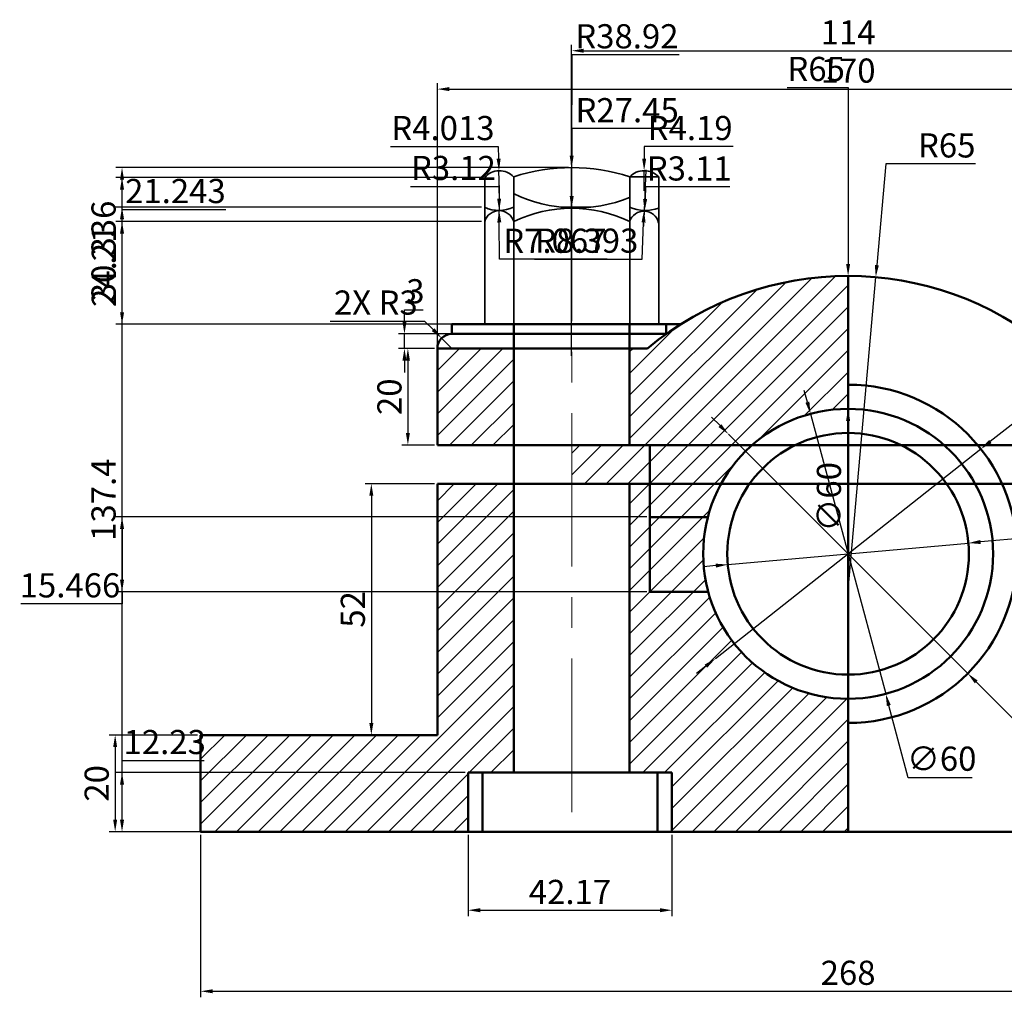
# Model space of a CAD drawing. Units: millimetres. Extents: x 2310 to 2633, y 1180 to 1382.
# Tile 1 of 2: x 2310 to 2514, y 1180 to 1382. Entities that reach past the tile are written whole.
import ezdxf

# ---------------------------------------------------------------- set-up
doc = ezdxf.new("R2010")
doc.units = ezdxf.units.MM
doc.linetypes.add('CENTER', pattern=[50.8, 31.75, -6.35, 6.35, -6.35])
for name, color, linetype, lineweight in [('M-CNTR', 1, 'CENTER', 18), ('M-DIMS', 2, 'Continuous', 25), ('M-FAST', 4, 'Continuous', 35), ('M-HATC', 8, 'Continuous', 18), ('M-OUTL', 7, 'Continuous', 50)]:
    doc.layers.add(name, color=color, linetype=linetype, lineweight=lineweight)
doc.styles.get("Standard").update_dxf_attribs({"font": 'arial.ttf'})
doc.dimstyles.new('ISO-25', dxfattribs={"dimtxt": 5, "dimasz": 2.5, "dimexe": 1.25, "dimexo": 0.625, "dimtad": 1, "dimtoh": 1, "dimdec": 0, "dimtxsty": 'Standard', "dimcen": 2.5, "dimadec": 0, "dimazin": 0, "dimtfac": 1, "dimtdec": 0, "dimtmove": 0, "dimatfit": 3, "dimfxl": 1, "dimarcsym": 0})

# ---------------------------------------------------------------- blocks, each defined once
blk = doc.blocks.new('*D1')
at = {"layer": 'Defpoints', "color": 0, "transparency": 16777216}
for p in [(2538.53, 1375.88), (2424.11, 1351.69), (2538.53, 1351.69)]:
    blk.add_point(p, dxfattribs=at)
at = {"layer": 'M-DIMS', "color": 0, "lineweight": -2, "transparency": 16777216}
for p, q in [((2424.11, 1352.31), (2424.11, 1377.13)), ((2426.61, 1375.88), (2536.03, 1375.88)), ((2538.53, 1352.31), (2538.53, 1377.13))]:
    blk.add_line(p, q, dxfattribs=at)
at = {"layer": 'M-DIMS', "color": 0, "transparency": 16777216}
for points in [[(2426.61, 1376.3), (2426.61, 1375.47), (2424.11, 1375.88)], [(2536.03, 1376.3), (2536.03, 1375.47), (2538.53, 1375.88)]]:
    blk.add_solid(points, dxfattribs=at)
at = {"layer": 'M-DIMS', "color": 0, "transparency": 16777216, "insert": (2481.32, 1379.02), "char_height": 5, "attachment_point": 5}
blk.add_mtext('114', dxfattribs=at)
blk = doc.blocks.new('*D2')
at = {"layer": 'Defpoints', "color": 0, "transparency": 16777216}
for p in [(2347.32, 1214.28), (2615.32, 1214.28), (2615.32, 1181.26)]:
    blk.add_point(p, dxfattribs=at)
at = {"layer": 'M-DIMS', "color": 0, "lineweight": -2, "transparency": 16777216}
for p, q in [((2347.32, 1213.66), (2347.32, 1180.01)), ((2615.32, 1213.66), (2615.32, 1180.01)), ((2349.82, 1181.26), (2612.82, 1181.26))]:
    blk.add_line(p, q, dxfattribs=at)
at = {"layer": 'M-DIMS', "color": 0, "transparency": 16777216}
for points in [[(2349.82, 1181.68), (2349.82, 1180.85), (2347.32, 1181.26)], [(2612.82, 1181.68), (2612.82, 1180.85), (2615.32, 1181.26)]]:
    blk.add_solid(points, dxfattribs=at)
at = {"layer": 'M-DIMS', "color": 0, "transparency": 16777216, "insert": (2481.32, 1184.44), "char_height": 5, "attachment_point": 5}
blk.add_mtext('268', dxfattribs=at)
blk = doc.blocks.new('*D3')
at = {"layer": 'Defpoints', "color": 0, "transparency": 16777216}
for p in [(2396.32, 1314.28), (2390.22, 1294.28), (2396.32, 1294.28)]:
    blk.add_point(p, dxfattribs=at)
at = {"layer": 'M-DIMS', "color": 0, "lineweight": -2, "transparency": 16777216}
for p, q in [((2395.7, 1314.28), (2388.97, 1314.28)), ((2390.22, 1311.78), (2390.22, 1296.78)), ((2395.7, 1294.28), (2388.97, 1294.28))]:
    blk.add_line(p, q, dxfattribs=at)
at = {"layer": 'M-DIMS', "color": 0, "transparency": 16777216}
for points in [[(2389.81, 1311.78), (2390.64, 1311.78), (2390.22, 1314.28)], [(2389.81, 1296.78), (2390.64, 1296.78), (2390.22, 1294.28)]]:
    blk.add_solid(points, dxfattribs=at)
at = {"layer": 'M-DIMS', "color": 0, "transparency": 16777216, "insert": (2387.05, 1304.28), "char_height": 5, "attachment_point": 5, "rotation": 90}
blk.add_mtext('20', dxfattribs=at)
blk = doc.blocks.new('*D4')
at = {"layer": 'Defpoints', "color": 0, "transparency": 16777216}
for p in [(2396.32, 1286.28), (2382.66, 1234.28), (2396.32, 1234.28)]:
    blk.add_point(p, dxfattribs=at)
at = {"layer": 'M-DIMS', "color": 0, "lineweight": -2, "transparency": 16777216}
for p, q in [((2395.7, 1286.28), (2381.41, 1286.28)), ((2382.66, 1283.78), (2382.66, 1236.78)), ((2395.7, 1234.28), (2381.41, 1234.28))]:
    blk.add_line(p, q, dxfattribs=at)
at = {"layer": 'M-DIMS', "color": 0, "transparency": 16777216}
for points in [[(2382.24, 1283.78), (2383.08, 1283.78), (2382.66, 1286.28)], [(2382.24, 1236.78), (2383.08, 1236.78), (2382.66, 1234.28)]]:
    blk.add_solid(points, dxfattribs=at)
at = {"layer": 'M-DIMS', "color": 0, "transparency": 16777216, "insert": (2379.48, 1260.28), "char_height": 5, "attachment_point": 5, "rotation": 90}
blk.add_mtext('52', dxfattribs=at)
blk = doc.blocks.new('*D5')
at = {"layer": 'Defpoints', "color": 0, "transparency": 16777216}
for p in [(2347.32, 1234.28), (2329.65, 1214.28), (2347.32, 1214.28)]:
    blk.add_point(p, dxfattribs=at)
at = {"layer": 'M-DIMS', "color": 0, "lineweight": -2, "transparency": 16777216}
for p, q in [((2346.7, 1234.28), (2328.4, 1234.28)), ((2329.65, 1231.78), (2329.65, 1216.78)), ((2346.7, 1214.28), (2328.4, 1214.28))]:
    blk.add_line(p, q, dxfattribs=at)
at = {"layer": 'M-DIMS', "color": 0, "transparency": 16777216}
for points in [[(2329.23, 1231.78), (2330.06, 1231.78), (2329.65, 1234.28)], [(2329.23, 1216.78), (2330.06, 1216.78), (2329.65, 1214.28)]]:
    blk.add_solid(points, dxfattribs=at)
at = {"layer": 'M-DIMS', "color": 0, "transparency": 16777216, "insert": (2326.47, 1224.28), "char_height": 5, "attachment_point": 5, "rotation": 90}
blk.add_mtext('20', dxfattribs=at)
blk = doc.blocks.new('*D6')
at = {"layer": 'Defpoints', "color": 0, "transparency": 16777216}
for p in [(2389.51, 1317.28), (2399.32, 1317.28), (2396.32, 1314.28)]:
    blk.add_point(p, dxfattribs=at)
at = {"layer": 'M-DIMS', "color": 0, "lineweight": -2, "transparency": 16777216}
for p, q in [((2389.51, 1319.78), (2389.51, 1322.28)), ((2389.51, 1322.28), (2393.41, 1322.28)), ((2398.7, 1317.28), (2388.26, 1317.28)), ((2389.51, 1314.28), (2389.51, 1317.28)), ((2395.7, 1314.28), (2388.26, 1314.28)), ((2389.51, 1311.78), (2389.51, 1309.28))]:
    blk.add_line(p, q, dxfattribs=at)
at = {"layer": 'M-DIMS', "color": 0, "transparency": 16777216}
for points in [[(2389.1, 1319.78), (2389.93, 1319.78), (2389.51, 1317.28)], [(2389.1, 1311.78), (2389.93, 1311.78), (2389.51, 1314.28)]]:
    blk.add_solid(points, dxfattribs=at)
at = {"layer": 'M-DIMS', "color": 0, "transparency": 16777216, "insert": (2391.78, 1325.46), "char_height": 5, "attachment_point": 5}
blk.add_mtext('3', dxfattribs=at)
blk = doc.blocks.new('*D8')
at = {"layer": 'Defpoints', "color": 0, "transparency": 16777216}
for p in [(2487.04, 1329.03), (2481.32, 1264.28)]:
    blk.add_point(p, dxfattribs=at)
at = {"layer": 'M-DIMS', "color": 0, "lineweight": -2, "transparency": 16777216}
for p, q in [((2489.11, 1352.46), (2487.26, 1331.52)), ((2507.71, 1352.46), (2489.11, 1352.46)), ((2481.32, 1264.28), (2487.04, 1329.03))]:
    blk.add_line(p, q, dxfattribs=at)
at = {"layer": 'M-DIMS', "color": 0, "transparency": 16777216}
blk.add_solid([(2486.85, 1331.56), (2487.68, 1331.48), (2487.04, 1329.03)], dxfattribs=at)
at = {"layer": 'M-DIMS', "color": 0, "transparency": 16777216, "insert": (2501.72, 1355.64), "char_height": 5, "attachment_point": 5}
blk.add_mtext('R65', dxfattribs=at)
blk = doc.blocks.new('*D9')
at = {"layer": 'Defpoints', "color": 0, "transparency": 16777216}
for p in [(2508.79, 1293.47), (2453.85, 1250.09)]:
    blk.add_point(p, dxfattribs=at)
at = {"layer": 'M-DIMS', "color": 0, "lineweight": -2, "transparency": 16777216}
for p, q in [((2516.9, 1299.87), (2510.75, 1295.02)), ((2536.4, 1299.87), (2516.9, 1299.87)), ((2453.85, 1250.09), (2508.79, 1293.47)), ((2451.89, 1248.54), (2449.93, 1246.99))]:
    blk.add_line(p, q, dxfattribs=at)
at = {"layer": 'M-DIMS', "color": 0, "transparency": 16777216}
for points in [[(2510.49, 1295.35), (2511.01, 1294.69), (2508.79, 1293.47)], [(2451.63, 1248.87), (2452.15, 1248.21), (2453.85, 1250.09)]]:
    blk.add_solid(points, dxfattribs=at)
at = {"layer": 'M-DIMS', "color": 0, "transparency": 16777216, "insert": (2530.11, 1303.19), "char_height": 5, "attachment_point": 5}
blk.add_mtext('∅70', dxfattribs=at)
blk = doc.blocks.new('*D10')
at = {"layer": 'Defpoints', "color": 0, "transparency": 16777216}
for p in [(2481.32, 1301.78), (2481.32, 1241.78)]:
    blk.add_point(p, dxfattribs=at)
at = {"layer": 'M-DIMS', "color": 0, "lineweight": -2, "transparency": 16777216}
blk.add_line((2481.32, 1276.65), (2481.32, 1299.28), dxfattribs=at)
at = {"layer": 'M-DIMS', "color": 0, "transparency": 16777216}
blk.add_solid([(2480.9, 1299.28), (2481.74, 1299.28), (2481.32, 1301.78)], dxfattribs=at)
at = {"layer": 'M-DIMS', "color": 0, "transparency": 16777216, "insert": (2478, 1283.57), "char_height": 5, "attachment_point": 5, "rotation": 90}
blk.add_mtext('∅60', dxfattribs=at)
blk = doc.blocks.new('*D11')
at = {"layer": 'Defpoints', "color": 0, "transparency": 16777216}
for p in [(2506.22, 1274.01), (2456.42, 1269.55)]:
    blk.add_point(p, dxfattribs=at)
at = {"layer": 'M-DIMS', "color": 0, "lineweight": -2, "transparency": 16777216}
for p, q in [((2456.42, 1269.55), (2506.22, 1274.01)), ((2520.89, 1275.32), (2508.71, 1274.23)), ((2534.1, 1275.32), (2520.89, 1275.32)), ((2453.93, 1269.33), (2451.44, 1269.11))]:
    blk.add_line(p, q, dxfattribs=at)
at = {"layer": 'M-DIMS', "color": 0, "transparency": 16777216}
for points in [[(2508.68, 1274.64), (2508.75, 1273.81), (2506.22, 1274.01)], [(2453.89, 1269.75), (2453.97, 1268.92), (2456.42, 1269.55)]]:
    blk.add_solid(points, dxfattribs=at)
at = {"layer": 'M-DIMS', "color": 0, "transparency": 16777216, "insert": (2527.81, 1278.64), "char_height": 5, "attachment_point": 5}
blk.add_mtext('∅50', dxfattribs=at)
blk = doc.blocks.new('HEX-NUT-M16')
for p, q in [((0.01, 21.24), (0.01, 30.34)), ((6.01, 27.03), (6.01, 30.51)), ((30.01, 30.51), (36.01, 30.51)), ((30.01, 28.24), (30.01, 30.51)), ((36.01, 28), (36.01, 30.51)), ((6.01, 24.24), (6.01, 27.03)), ((30.01, 24.24), (30.01, 28.24)), ((36.01, 24), (36.01, 28)), ((6.01, 21.24), (6.01, 24.24)), ((22, 24.24), (15.78, 24.24)), ((30.01, 21.24), (30.01, 24.24)), ((36.01, 21), (36.01, 24)), ((0.01, 0), (0.01, 21.24)), ((6.01, 21.24), (6.01, 0)), ((30.01, 21.24), (30.01, 0)), ((36.01, 0), (36.01, 21)), ((6.01, 0), (0.01, 0)), ((30.01, 0), (36.01, 0))]:
    blk.add_line(p, q)
for centre, radius, start, end in [((3.08, 27.76), 4.01, 43.2858, 140.0947), ((18.01, -6.51), 38.92, 72.0429, 107.9571), ((33.01, 27.59), 4.19, 44.2799, 135.7201), ((18.89, 53.7), 29.62, 244.2052, 292.0376), ((2.96, 30.62), 7.07, 245.1977, 295.4854), ((3.01, 20.39), 3.12, 15.8422, 164.1674), ((18.01, -3.45), 27.45, 64.08, 115.92), ((33.32, 31.95), 8.39, 246.714, 288.6385), ((32.97, 20.31), 3.11, 12.8097, 162.5427)]:
    blk.add_arc(centre, radius, start, end)
blk = doc.blocks.new('*D13')
at = {"layer": 'Defpoints', "color": 0, "transparency": 16777216}
for p in [(2566.32, 1367.94), (2396.32, 1314.28), (2566.32, 1314.28)]:
    blk.add_point(p, dxfattribs=at)
at = {"layer": 'M-DIMS', "color": 0, "lineweight": -2, "transparency": 16777216}
for p, q in [((2396.32, 1314.91), (2396.32, 1369.19)), ((2398.82, 1367.94), (2563.82, 1367.94)), ((2566.32, 1314.91), (2566.32, 1369.19))]:
    blk.add_line(p, q, dxfattribs=at)
at = {"layer": 'M-DIMS', "color": 0, "transparency": 16777216}
for points in [[(2398.82, 1368.36), (2398.82, 1367.52), (2396.32, 1367.94)], [(2563.82, 1368.36), (2563.82, 1367.52), (2566.32, 1367.94)]]:
    blk.add_solid(points, dxfattribs=at)
at = {"layer": 'M-DIMS', "color": 0, "transparency": 16777216, "insert": (2481.32, 1371.12), "char_height": 5, "attachment_point": 5}
blk.add_mtext('170', dxfattribs=at)
blk = doc.blocks.new('*D16')
at = {"layer": 'Defpoints', "color": 0, "transparency": 16777216}
for p in [(2331.07, 1351.69), (2424.11, 1351.69), (2347.32, 1214.28)]:
    blk.add_point(p, dxfattribs=at)
at = {"layer": 'M-DIMS', "color": 0, "lineweight": -2, "transparency": 16777216}
for p, q in [((2423.49, 1351.69), (2329.82, 1351.69)), ((2331.07, 1216.78), (2331.07, 1349.19)), ((2346.7, 1214.28), (2329.82, 1214.28))]:
    blk.add_line(p, q, dxfattribs=at)
at = {"layer": 'M-DIMS', "color": 0, "transparency": 16777216}
for points in [[(2330.65, 1349.19), (2331.49, 1349.19), (2331.07, 1351.69)], [(2330.65, 1216.78), (2331.49, 1216.78), (2331.07, 1214.28)]]:
    blk.add_solid(points, dxfattribs=at)
at = {"layer": 'M-DIMS', "color": 0, "transparency": 16777216, "insert": (2327.89, 1282.98), "char_height": 5, "attachment_point": 5, "rotation": 90}
blk.add_mtext('137.4', dxfattribs=at)
blk = doc.blocks.new('*D17')
at = {"layer": 'Defpoints', "color": 0, "transparency": 16777216}
for p in [(2402.68, 1214.28), (2444.86, 1214.28), (2444.86, 1198.03)]:
    blk.add_point(p, dxfattribs=at)
at = {"layer": 'M-DIMS', "color": 0, "lineweight": -2, "transparency": 16777216}
for p, q in [((2402.68, 1213.66), (2402.68, 1196.78)), ((2444.86, 1213.66), (2444.86, 1196.78)), ((2405.18, 1198.03), (2442.36, 1198.03))]:
    blk.add_line(p, q, dxfattribs=at)
at = {"layer": 'M-DIMS', "color": 0, "transparency": 16777216}
for points in [[(2405.18, 1198.45), (2405.18, 1197.61), (2402.68, 1198.03)], [(2442.36, 1198.45), (2442.36, 1197.61), (2444.86, 1198.03)]]:
    blk.add_solid(points, dxfattribs=at)
at = {"layer": 'M-DIMS', "color": 0, "transparency": 16777216, "insert": (2423.77, 1201.17), "char_height": 5, "attachment_point": 5}
blk.add_mtext('42.17', dxfattribs=at)
blk = doc.blocks.new('*D18')
at = {"layer": 'Defpoints', "color": 0, "transparency": 16777216}
for p in [(2331.07, 1226.51), (2402.68, 1226.51), (2402.68, 1214.28)]:
    blk.add_point(p, dxfattribs=at)
at = {"layer": 'M-DIMS', "color": 0, "lineweight": -2, "transparency": 16777216}
for p, q in [((2331.07, 1226.51), (2331.07, 1229.01)), ((2331.07, 1229.01), (2348.1, 1229.01)), ((2402.06, 1226.51), (2329.82, 1226.51)), ((2331.07, 1216.78), (2331.07, 1224.01)), ((2402.06, 1214.28), (2329.82, 1214.28))]:
    blk.add_line(p, q, dxfattribs=at)
at = {"layer": 'M-DIMS', "color": 0, "transparency": 16777216}
for points in [[(2330.65, 1224.01), (2331.49, 1224.01), (2331.07, 1226.51)], [(2330.65, 1216.78), (2331.49, 1216.78), (2331.07, 1214.28)]]:
    blk.add_solid(points, dxfattribs=at)
at = {"layer": 'M-DIMS', "color": 0, "transparency": 16777216, "insert": (2339.9, 1232.19), "char_height": 5, "attachment_point": 5}
blk.add_mtext('12.23', dxfattribs=at)
blk = doc.blocks.new('*D19')
at = {"layer": 'Defpoints', "color": 0, "transparency": 16777216}
for p in [(2473.54, 1300.75), (2489.1, 1242.81)]:
    blk.add_point(p, dxfattribs=at)
at = {"layer": 'M-DIMS', "color": 0, "lineweight": -2, "transparency": 16777216}
for p, q in [((2472.9, 1303.17), (2472.25, 1305.58)), ((2473.54, 1300.75), (2489.1, 1242.81)), ((2493.76, 1225.42), (2489.75, 1240.39)), ((2506.97, 1225.42), (2493.76, 1225.42))]:
    blk.add_line(p, q, dxfattribs=at)
at = {"layer": 'M-DIMS', "color": 0, "transparency": 16777216}
for points in [[(2473.3, 1303.28), (2472.49, 1303.06), (2473.54, 1300.75)], [(2490.15, 1240.5), (2489.34, 1240.28), (2489.1, 1242.81)]]:
    blk.add_solid(points, dxfattribs=at)
at = {"layer": 'M-DIMS', "color": 0, "transparency": 16777216, "insert": (2500.68, 1228.74), "char_height": 5, "attachment_point": 5}
blk.add_mtext('∅60', dxfattribs=at)
blk = doc.blocks.new('*D20')
at = {"layer": 'Defpoints', "color": 0, "transparency": 16777216}
for p in [(2456.57, 1296.53), (2506.07, 1247.03)]:
    blk.add_point(p, dxfattribs=at)
at = {"layer": 'M-DIMS', "color": 0, "lineweight": -2, "transparency": 16777216}
for p, q in [((2454.81, 1298.3), (2453.04, 1300.07)), ((2456.57, 1296.53), (2506.07, 1247.03)), ((2520.92, 1232.18), (2507.84, 1245.26)), ((2534.13, 1232.18), (2520.92, 1232.18))]:
    blk.add_line(p, q, dxfattribs=at)
at = {"layer": 'M-DIMS', "color": 0, "transparency": 16777216}
for points in [[(2455.1, 1298.59), (2454.51, 1298), (2456.57, 1296.53)], [(2508.13, 1245.56), (2507.54, 1244.97), (2506.07, 1247.03)]]:
    blk.add_solid(points, dxfattribs=at)
at = {"layer": 'M-DIMS', "color": 0, "transparency": 16777216, "insert": (2527.84, 1235.5), "char_height": 5, "attachment_point": 5}
blk.add_mtext('∅70', dxfattribs=at)
blk = doc.blocks.new('*D21')
at = {"layer": 'Defpoints', "color": 0, "transparency": 16777216}
for p in [(2481.32, 1329.28), (2481.32, 1264.28)]:
    blk.add_point(p, dxfattribs=at)
at = {"layer": 'M-DIMS', "color": 0, "lineweight": -2, "transparency": 16777216}
for p, q in [((2468.71, 1368.28), (2481.32, 1368.28)), ((2481.32, 1368.28), (2481.32, 1331.78)), ((2481.32, 1264.28), (2481.32, 1329.28))]:
    blk.add_line(p, q, dxfattribs=at)
at = {"layer": 'M-DIMS', "color": 0, "transparency": 16777216}
blk.add_solid([(2481.74, 1331.78), (2480.9, 1331.78), (2481.32, 1329.28)], dxfattribs=at)
at = {"layer": 'M-DIMS', "color": 0, "transparency": 16777216, "insert": (2474.7, 1371.46), "char_height": 5, "attachment_point": 5}
blk.add_mtext('R65', dxfattribs=at)
blk = doc.blocks.new('*D23')
at = {"layer": 'Defpoints', "color": 0, "transparency": 16777216}
for p in [(2397.2, 1316.4), (2399.32, 1314.28)]:
    blk.add_point(p, dxfattribs=at)
at = {"layer": 'M-DIMS', "color": 0, "lineweight": -2, "transparency": 16777216}
for p, q in [((2374.15, 1319.94), (2393.66, 1319.94)), ((2393.66, 1319.94), (2395.43, 1318.17)), ((2399.32, 1314.28), (2397.2, 1316.4))]:
    blk.add_line(p, q, dxfattribs=at)
at = {"layer": 'M-DIMS', "color": 0, "transparency": 16777216}
blk.add_solid([(2395.73, 1318.46), (2395.14, 1317.88), (2397.2, 1316.4)], dxfattribs=at)
at = {"layer": 'M-DIMS', "color": 0, "transparency": 16777216, "insert": (2383.59, 1323.12), "char_height": 5, "attachment_point": 5}
blk.add_mtext('2X R3', dxfattribs=at)
blk = doc.blocks.new('*D25')
at = {"layer": 'Defpoints', "color": 0, "transparency": 16777216}
for p in [(2331.07, 1340.52), (2406.11, 1340.52), (2406.11, 1319.28)]:
    blk.add_point(p, dxfattribs=at)
at = {"layer": 'M-DIMS', "color": 0, "lineweight": -2, "transparency": 16777216}
for p, q in [((2331.07, 1340.52), (2331.07, 1343.02)), ((2331.07, 1343.02), (2352.54, 1343.02)), ((2405.49, 1340.52), (2329.82, 1340.52)), ((2331.07, 1321.78), (2331.07, 1338.02)), ((2405.49, 1319.28), (2329.82, 1319.28))]:
    blk.add_line(p, q, dxfattribs=at)
at = {"layer": 'M-DIMS', "color": 0, "transparency": 16777216}
for points in [[(2330.65, 1338.02), (2331.49, 1338.02), (2331.07, 1340.52)], [(2330.65, 1321.78), (2331.49, 1321.78), (2331.07, 1319.28)]]:
    blk.add_solid(points, dxfattribs=at)
at = {"layer": 'M-DIMS', "color": 0, "transparency": 16777216, "insert": (2342.12, 1346.2), "char_height": 5, "attachment_point": 5}
blk.add_mtext('21.243', dxfattribs=at)
blk = doc.blocks.new('*D26')
at = {"layer": 'Defpoints', "color": 0, "transparency": 16777216}
for p in [(2331.07, 1343.49), (2406.11, 1343.49), (2406.11, 1319.28)]:
    blk.add_point(p, dxfattribs=at)
at = {"layer": 'M-DIMS', "color": 0, "lineweight": -2, "transparency": 16777216}
for p, q in [((2405.48, 1343.49), (2329.82, 1343.49)), ((2331.07, 1321.78), (2331.07, 1340.99)), ((2405.49, 1319.28), (2329.82, 1319.28))]:
    blk.add_line(p, q, dxfattribs=at)
at = {"layer": 'M-DIMS', "color": 0, "transparency": 16777216}
for points in [[(2330.65, 1340.99), (2331.49, 1340.99), (2331.07, 1343.49)], [(2330.65, 1321.78), (2331.49, 1321.78), (2331.07, 1319.28)]]:
    blk.add_solid(points, dxfattribs=at)
at = {"layer": 'M-DIMS', "color": 0, "transparency": 16777216, "insert": (2327.94, 1331.38), "char_height": 5, "attachment_point": 5, "rotation": 90}
blk.add_mtext('24.21', dxfattribs=at)
blk = doc.blocks.new('*D27')
at = {"layer": 'Defpoints', "color": 0, "transparency": 16777216}
for p in [(2331.07, 1349.62), (2406.11, 1349.62), (2406.11, 1319.28)]:
    blk.add_point(p, dxfattribs=at)
at = {"layer": 'M-DIMS', "color": 0, "lineweight": -2, "transparency": 16777216}
for p, q in [((2405.49, 1349.62), (2329.82, 1349.62)), ((2331.07, 1321.78), (2331.07, 1347.12)), ((2405.49, 1319.28), (2329.82, 1319.28))]:
    blk.add_line(p, q, dxfattribs=at)
at = {"layer": 'M-DIMS', "color": 0, "transparency": 16777216}
for points in [[(2330.65, 1347.12), (2331.49, 1347.12), (2331.07, 1349.62)], [(2330.65, 1321.78), (2331.49, 1321.78), (2331.07, 1319.28)]]:
    blk.add_solid(points, dxfattribs=at)
at = {"layer": 'M-DIMS', "color": 0, "transparency": 16777216, "insert": (2327.89, 1334.45), "char_height": 5, "attachment_point": 5, "rotation": 90}
blk.add_mtext('30.336', dxfattribs=at)
blk = doc.blocks.new('*D28')
at = {"layer": 'Defpoints', "color": 0, "transparency": 16777216}
for p in [(2440.28, 1279.4), (2331.07, 1263.93), (2440.28, 1263.93)]:
    blk.add_point(p, dxfattribs=at)
at = {"layer": 'M-DIMS', "color": 0, "lineweight": -2, "transparency": 16777216}
for p, q in [((2439.65, 1279.4), (2329.82, 1279.4)), ((2331.07, 1276.9), (2331.07, 1266.43)), ((2439.65, 1263.93), (2329.82, 1263.93)), ((2331.07, 1263.93), (2331.07, 1261.43)), ((2331.07, 1261.43), (2310.16, 1261.43))]:
    blk.add_line(p, q, dxfattribs=at)
at = {"layer": 'M-DIMS', "color": 0, "transparency": 16777216}
for points in [[(2330.65, 1276.9), (2331.49, 1276.9), (2331.07, 1279.4)], [(2330.65, 1266.43), (2331.49, 1266.43), (2331.07, 1263.93)]]:
    blk.add_solid(points, dxfattribs=at)
at = {"layer": 'M-DIMS', "color": 0, "transparency": 16777216, "insert": (2320.3, 1264.61), "char_height": 5, "attachment_point": 5}
blk.add_mtext('15.466', dxfattribs=at)
blk = doc.blocks.new('*D29')
at = {"layer": 'Defpoints', "color": 0, "transparency": 16777216}
for p in [(2424.11, 1351.69), (2424.11, 1312.77)]:
    blk.add_point(p, dxfattribs=at)
at = {"layer": 'M-DIMS', "color": 0, "lineweight": -2, "transparency": 16777216}
for p, q in [((2446.35, 1375.04), (2424.12, 1375.04)), ((2424.12, 1375.04), (2424.11, 1354.19)), ((2424.11, 1312.77), (2424.11, 1351.69))]:
    blk.add_line(p, q, dxfattribs=at)
at = {"layer": 'M-DIMS', "color": 0, "transparency": 16777216}
blk.add_solid([(2423.7, 1354.19), (2424.53, 1354.19), (2424.11, 1351.69)], dxfattribs=at)
at = {"layer": 'M-DIMS', "color": 0, "transparency": 16777216, "insert": (2435.54, 1378.22), "char_height": 5, "attachment_point": 5}
blk.add_mtext('R38.92', dxfattribs=at)
blk = doc.blocks.new('*D30')
at = {"layer": 'Defpoints', "color": 0, "transparency": 16777216}
for p in [(2424.11, 1343.29), (2424.11, 1315.83)]:
    blk.add_point(p, dxfattribs=at)
at = {"layer": 'M-DIMS', "color": 0, "lineweight": -2, "transparency": 16777216}
for p, q in [((2446.44, 1359.76), (2424.12, 1359.76)), ((2424.12, 1359.76), (2424.11, 1345.79)), ((2424.11, 1315.83), (2424.11, 1343.29))]:
    blk.add_line(p, q, dxfattribs=at)
at = {"layer": 'M-DIMS', "color": 0, "transparency": 16777216}
blk.add_solid([(2423.7, 1345.79), (2424.53, 1345.79), (2424.11, 1343.29)], dxfattribs=at)
at = {"layer": 'M-DIMS', "color": 0, "transparency": 16777216, "insert": (2435.59, 1362.93), "char_height": 5, "attachment_point": 5}
blk.add_mtext('R27.45', dxfattribs=at)
blk = doc.blocks.new('*D31')
at = {"layer": 'Defpoints', "color": 0, "transparency": 16777216}
for p in [(2439.43, 1351.23), (2439.09, 1342.85)]:
    blk.add_point(p, dxfattribs=at)
at = {"layer": 'M-DIMS', "color": 0, "lineweight": -2, "transparency": 16777216}
for p, q in [((2439.43, 1351.23), (2439.09, 1342.85)), ((2438.68, 1332.75), (2438.99, 1340.35)), ((2416.4, 1332.75), (2438.68, 1332.75))]:
    blk.add_line(p, q, dxfattribs=at)
at = {"layer": 'M-DIMS', "color": 0, "transparency": 16777216}
blk.add_solid([(2438.57, 1340.37), (2439.41, 1340.33), (2439.09, 1342.85)], dxfattribs=at)
at = {"layer": 'M-DIMS', "color": 0, "transparency": 16777216, "insert": (2427.23, 1335.93), "char_height": 5, "attachment_point": 5}
blk.add_mtext('R8.393', dxfattribs=at)
blk = doc.blocks.new('*D32')
at = {"layer": 'Defpoints', "color": 0, "transparency": 16777216}
for p in [(2409.07, 1349.9), (2409.12, 1342.84)]:
    blk.add_point(p, dxfattribs=at)
at = {"layer": 'M-DIMS', "color": 0, "lineweight": -2, "transparency": 16777216}
for p, q in [((2409.07, 1349.9), (2409.12, 1342.84)), ((2409.18, 1332.73), (2409.13, 1340.34)), ((2431.46, 1332.73), (2409.18, 1332.73))]:
    blk.add_line(p, q, dxfattribs=at)
at = {"layer": 'M-DIMS', "color": 0, "transparency": 16777216}
blk.add_solid([(2409.55, 1340.34), (2408.71, 1340.33), (2409.12, 1342.84)], dxfattribs=at)
at = {"layer": 'M-DIMS', "color": 0, "transparency": 16777216, "insert": (2420.63, 1335.91), "char_height": 5, "attachment_point": 5}
blk.add_mtext('R7.067', dxfattribs=at)
blk = doc.blocks.new('*D33')
at = {"layer": 'Defpoints', "color": 0, "transparency": 16777216}
for p in [(2439.11, 1351.06), (2439.11, 1346.87)]:
    blk.add_point(p, dxfattribs=at)
at = {"layer": 'M-DIMS', "color": 0, "lineweight": -2, "transparency": 16777216}
for p, q in [((2457.52, 1356.06), (2439.12, 1356.06)), ((2439.12, 1356.06), (2439.12, 1353.56)), ((2439.11, 1346.87), (2439.11, 1351.06))]:
    blk.add_line(p, q, dxfattribs=at)
at = {"layer": 'M-DIMS', "color": 0, "transparency": 16777216}
blk.add_solid([(2438.7, 1353.56), (2439.53, 1353.56), (2439.11, 1351.06)], dxfattribs=at)
at = {"layer": 'M-DIMS', "color": 0, "transparency": 16777216, "insert": (2448.63, 1359.24), "char_height": 5, "attachment_point": 5}
blk.add_mtext('R4.19', dxfattribs=at)
blk = doc.blocks.new('*D34')
at = {"layer": 'Defpoints', "color": 0, "transparency": 16777216}
for p in [(2409.07, 1351.05), (2409.19, 1347.04)]:
    blk.add_point(p, dxfattribs=at)
at = {"layer": 'M-DIMS', "color": 0, "lineweight": -2, "transparency": 16777216}
for p, q in [((2386.65, 1356.05), (2408.93, 1356.05)), ((2408.93, 1356.05), (2409, 1353.55)), ((2409.19, 1347.04), (2409.07, 1351.05))]:
    blk.add_line(p, q, dxfattribs=at)
at = {"layer": 'M-DIMS', "color": 0, "transparency": 16777216}
blk.add_solid([(2409.42, 1353.56), (2408.58, 1353.54), (2409.07, 1351.05)], dxfattribs=at)
at = {"layer": 'M-DIMS', "color": 0, "transparency": 16777216, "insert": (2397.47, 1359.23), "char_height": 5, "attachment_point": 5}
blk.add_mtext('R4.013', dxfattribs=at)
blk = doc.blocks.new('*D35')
at = {"layer": 'Defpoints', "color": 0, "transparency": 16777216}
for p in [(2409.11, 1342.79), (2409.11, 1339.67)]:
    blk.add_point(p, dxfattribs=at)
at = {"layer": 'M-DIMS', "color": 0, "lineweight": -2, "transparency": 16777216}
for p, q in [((2390.77, 1347.79), (2409.11, 1347.79)), ((2409.11, 1347.79), (2409.11, 1345.29)), ((2409.11, 1339.67), (2409.11, 1342.79))]:
    blk.add_line(p, q, dxfattribs=at)
at = {"layer": 'M-DIMS', "color": 0, "transparency": 16777216}
blk.add_solid([(2409.53, 1345.29), (2408.7, 1345.29), (2409.11, 1342.79)], dxfattribs=at)
at = {"layer": 'M-DIMS', "color": 0, "transparency": 16777216, "insert": (2399.63, 1350.97), "char_height": 5, "attachment_point": 5}
blk.add_mtext('R3.12', dxfattribs=at)
blk = doc.blocks.new('*D36')
at = {"layer": 'Defpoints', "color": 0, "transparency": 16777216}
for p in [(2439.21, 1342.7), (2439.08, 1339.59)]:
    blk.add_point(p, dxfattribs=at)
at = {"layer": 'M-DIMS', "color": 0, "lineweight": -2, "transparency": 16777216}
for p, q in [((2439.41, 1347.69), (2439.31, 1345.2)), ((2456.84, 1347.69), (2439.41, 1347.69)), ((2439.08, 1339.59), (2439.21, 1342.7))]:
    blk.add_line(p, q, dxfattribs=at)
at = {"layer": 'M-DIMS', "color": 0, "transparency": 16777216}
blk.add_solid([(2438.89, 1345.21), (2439.73, 1345.18), (2439.21, 1342.7)], dxfattribs=at)
at = {"layer": 'M-DIMS', "color": 0, "transparency": 16777216, "insert": (2448.44, 1350.87), "char_height": 5, "attachment_point": 5}
blk.add_mtext('R3.11', dxfattribs=at)

msp = doc.modelspace()

# ---------------------------------------------------------------- hatches: boundary and pattern name
at = {"layer": 'M-HATC'}
h = msp.add_hatch(dxfattribs=at)
h.set_pattern_fill('ANSI31', color=256)
h.paths.add_polyline_path([(2481.3215, 1329.2804, 0.17504567), (2439.7883, 1314.2804), (2436.1145, 1314.2804), (2436.1145, 1294.2804), (2461.4783, 1294.2804, -0.18267581), (2481.3215, 1301.7804)])
h.paths.add_polyline_path([(2481.3215, 1241.7804, -0.33862389), (2452.3669, 1263.9295), (2440.2782, 1263.9295), (2440.2782, 1279.3954), (2440.2782, 1286.2804), (2436.1145, 1286.2804), (2436.1145, 1226.5103), (2444.8583, 1226.5103), (2444.8583, 1214.2804), (2481.3215, 1214.2804)])
h.paths.add_polyline_path([(2452.304, 1279.3954), (2440.2782, 1279.3954), (2440.2782, 1263.9295), (2452.3669, 1263.9295, -0.06629146), (2451.3215, 1271.7804, -0.06424898)], flags=17)
h.paths.add_polyline_path([(2455.0584, 1286.2804), (2440.2782, 1286.2804), (2440.2782, 1279.3954), (2452.304, 1279.3954, -0.06203318)])
h.paths.add_polyline_path([(2461.4783, 1294.2804), (2440.2782, 1294.2804), (2440.2782, 1286.2804), (2455.0584, 1286.2804, -0.08611284)])
h.paths.add_polyline_path([(2440.2782, 1294.2804), (2436.1145, 1294.2804), (2424.1145, 1294.2804), (2424.1145, 1286.2804), (2440.2782, 1286.2804)])
h.paths.add_polyline_path([(2412.1145, 1286.2804), (2396.3215, 1286.2804), (2396.3215, 1234.2804), (2381.3215, 1234.2804), (2347.3215, 1234.2804), (2347.3215, 1214.2804), (2402.6841, 1214.2804), (2402.6841, 1226.5103), (2412.1145, 1226.5103)])
h.paths.add_polyline_path([(2412.1145, 1314.2804), (2396.3215, 1314.2804), (2396.3215, 1294.2804), (2412.1145, 1294.2804)])

# ---------------------------------------------------------------- linework, layer by layer
at = {"layer": 'M-CNTR'}
msp.add_line((2424.1145, 1351.6891), (2424.1145, 1214.2804), dxfattribs=at)
at = {"layer": 'M-OUTL'}
for p, q in [((2481.3215, 1329.2804), (2481.3215, 1214.2804)), ((2443.6917, 1319.2804), (2399.3215, 1319.2804)), ((2399.3215, 1317.2804), (2399.3215, 1319.2804)), ((2399.3215, 1319.2804), (2446.6804, 1319.2804)), ((2446.6804, 1319.2804), (2399.3215, 1319.2804)), ((2412.1145, 1319.2804), (2412.1145, 1226.5103)), ((2436.1145, 1319.2804), (2436.1145, 1294.2804)), ((2443.6917, 1317.2804), (2443.6917, 1319.2804)), ((2443.6917, 1317.2804), (2399.3215, 1317.2804)), ((2439.7883, 1314.2804), (2396.3215, 1314.2804)), ((2396.3215, 1314.2804), (2396.3215, 1314.2804)), ((2396.3215, 1314.2804), (2396.3215, 1294.2804)), ((2396.3215, 1294.2804), (2396.3215, 1314.2804)), ((2396.3215, 1294.2804), (2566.3215, 1294.2804)), ((2440.2782, 1279.3954), (2440.2782, 1294.2804)), ((2396.3215, 1234.2804), (2396.3215, 1286.2804)), ((2566.3215, 1286.2804), (2396.3215, 1286.2804)), ((2436.1145, 1286.2804), (2436.1145, 1226.5103)), ((2452.304, 1279.3954), (2440.2782, 1279.3954)), ((2440.2782, 1279.3954), (2440.2782, 1263.9295)), ((2452.3669, 1263.9295), (2440.2782, 1263.9295)), ((2347.3215, 1214.2804), (2347.3215, 1234.2804)), ((2347.3215, 1234.2804), (2381.3215, 1234.2804)), ((2381.3215, 1234.2804), (2396.3215, 1234.2804)), ((2402.6841, 1226.5103), (2444.8583, 1226.5103)), ((2402.6841, 1226.5103), (2402.6841, 1214.2804)), ((2405.6841, 1214.2804), (2405.6841, 1226.5103)), ((2441.8583, 1214.2804), (2441.8583, 1226.5103)), ((2444.8583, 1226.5103), (2444.8583, 1214.2804)), ((2347.3215, 1214.2804), (2615.3215, 1214.2804)), ((2402.6841, 1214.2804), (2405.6841, 1214.2804)), ((2444.8583, 1214.2804), (2441.8583, 1214.2804))]:
    msp.add_line(p, q, dxfattribs=at)
for radius in [30, 25]:
    msp.add_circle((2481.3215, 1271.7804), radius, dxfattribs=at)
for centre, radius, start, end in [((2481.3215, 1264.2804), 65, 50.284863, 129.715137), ((2399.3215, 1314.2804), 3, 90, 180), ((2481.3215, 1271.7804), 35, 270, 90)]:
    msp.add_arc(centre, radius, start, end, dxfattribs=at)

# ---------------------------------------------------------------- block references
at = {"layer": 'M-FAST'}
msp.add_blockref('HEX-NUT-M16', (2406.109, 1319.28), dxfattribs=at)

# ---------------------------------------------------------------- dimensions: what is measured, and where the dimension line sits
at = {"layer": 'M-DIMS'}
for center, mpoint, override, picture, middle in [((2424.1145, 1312.7667), (2424.115, 1351.6891), {"dimdec": 2, "dimlfac": 1, "dimrnd": 0, "dimzin": 0, "dimdsep": 46, "dimlunit": 2}, '*D29', (2435.5435, 1375.0426)), ((2481.3215, 1264.2804), (2481.321, 1329.2804), {"dimdec": 0, "dimlfac": 1, "dimrnd": 0, "dimzin": 0, "dimdsep": 46, "dimlunit": 2}, '*D21', (2474.7032, 1368.2804)), ((2424.1145, 1315.8327), (2424.115, 1343.2855), {"dimdec": 2, "dimlfac": 1, "dimrnd": 0, "dimzin": 0, "dimdsep": 46, "dimlunit": 2}, '*D30', (2435.5878, 1359.7571)), ((2481.3215, 1264.2804), (2487.0405, 1329.0283), {"dimclrd": 0, "dimclre": 0, "dimclrt": 0}, '*D8', (2501.7202, 1352.46))]:
    dim = msp.add_radius_dim(center=center, mpoint=mpoint, dimstyle='ISO-25', override=override, dxfattribs=at)
    dim.commit()
    dim.dimension.update_dxf_attribs({"geometry": picture, "text_midpoint": middle, "dimtype": 164})
for base, p1, p2, override, picture, middle in [((2538.5284, 1375.8841), (2424.1145, 1351.6891), (2538.5284, 1351.6891), {"dimclrd": 0, "dimclre": 0, "dimclrt": 0}, '*D1', (2481.3215, 1379.0193)), ((2566.3215, 1367.9391), (2396.3215, 1314.2804), (2566.3215, 1314.2804), {"dimdec": 0, "dimlfac": 1, "dimrnd": 0, "dimzin": 0, "dimdsep": 46, "dimlunit": 2}, '*D13', (2481.3215, 1371.117)), ((2615.3215, 1181.2637), (2347.3215, 1214.2804), (2615.3215, 1214.2804), {"dimclrd": 0, "dimclre": 0, "dimclrt": 0}, '*D2', (2481.3215, 1184.4416)), ((2444.8583, 1198.0304), (2402.6841, 1214.2804), (2444.8583, 1214.2804), {"dimdec": 2, "dimlfac": 1, "dimrnd": 0, "dimzin": 0, "dimdsep": 46, "dimlunit": 2}, '*D17', (2423.7712, 1201.1656))]:
    dim = msp.add_linear_dim(base=base, p1=p1, p2=p2, dimstyle='ISO-25', override=override, dxfattribs=at)
    dim.commit()
    dim.dimension.update_dxf_attribs({"geometry": picture, "text_midpoint": middle})
for center, mpoint, override, picture, middle in [((2409.1931, 1347.0415), (2409.075, 1351.053), {"dimdec": 3, "dimlfac": 1, "dimrnd": 0, "dimzin": 0, "dimdsep": 46, "dimlunit": 2}, '*D34', (2397.4741, 1359.2304)), ((2439.1145, 1346.8676), (2439.115, 1351.0579), {"dimdec": 2, "dimlfac": 1, "dimrnd": 0, "dimzin": 0, "dimdsep": 46, "dimlunit": 2}, '*D33', (2448.6321, 1359.2358)), ((2409.1146, 1339.6726), (2409.114, 1342.791), {"dimdec": 2, "dimlfac": 1, "dimrnd": 0, "dimzin": 0, "dimdsep": 46, "dimlunit": 2}, '*D35', (2399.6272, 1350.9705)), ((2439.0816, 1339.5908), (2439.208, 1342.6985), {"dimdec": 2, "dimlfac": 1, "dimrnd": 0, "dimzin": 0, "dimdsep": 46, "dimlunit": 2}, '*D36', (2448.44, 1350.874)), ((2439.4323, 1351.2328), (2439.092, 1342.8471), {"dimdec": 3, "dimlfac": 1, "dimrnd": 0, "dimzin": 0, "dimdsep": 46, "dimlunit": 2}, '*D31', (2427.2284, 1335.9259)), ((2409.0736, 1349.9034), (2409.116, 1342.8363), {"dimdec": 3, "dimlfac": 1, "dimrnd": 0, "dimzin": 0, "dimdsep": 46, "dimlunit": 2}, '*D32', (2420.6304, 1335.9086))]:
    dim = msp.add_radius_dim(center=center, mpoint=mpoint, dimstyle='ISO-25', override=override, dxfattribs=at)
    dim.commit()
    dim.dimension.update_dxf_attribs({"geometry": picture, "text_midpoint": middle})
for base, p1, p2, override, picture, middle in [((2331.0715, 1351.6891), (2347.3215, 1214.2804), (2424.1145, 1351.6891), {"dimdec": 1, "dimlfac": 1, "dimrnd": 0, "dimzin": 0, "dimdsep": 46, "dimlunit": 2}, '*D16', (2327.8919, 1282.9848)), ((2331.0715, 1349.6161), (2406.1145, 1319.2804), (2406.1145, 1349.6161), {"dimdec": 3, "dimlfac": 1, "dimrnd": 0, "dimzin": 0, "dimdsep": 46, "dimlunit": 2}, '*D27', (2327.8919, 1334.4482)), ((2331.0715, 1340.5234), (2406.1145, 1319.2804), (2406.1145, 1340.5234), {"dimdec": 3, "dimlfac": 1, "dimrnd": 0, "dimzin": 0, "dimdsep": 46, "dimlunit": 2}, '*D25', (2342.1177, 1346.2029)), ((2331.0715, 1343.4881), (2406.1145, 1319.2804), (2406.109, 1343.4881), {"dimdec": 2, "dimlfac": 1, "dimrnd": 0, "dimzin": 0, "dimdsep": 46, "dimlunit": 2}, '*D26', (2327.9362, 1331.3842)), ((2389.5133, 1317.2804), (2396.3215, 1314.2804), (2399.3215, 1317.2804), {"dimclrd": 0, "dimclre": 0, "dimclrt": 0}, '*D6', (2391.7754, 1325.46)), ((2390.2249, 1294.2804), (2396.3215, 1314.2804), (2396.3215, 1294.2804), {"dimclrd": 0, "dimclre": 0, "dimclrt": 0}, '*D3', (2387.047, 1304.2804)), ((2382.6602, 1234.2804), (2396.3215, 1286.2804), (2396.3215, 1234.2804), {"dimclrd": 0, "dimclre": 0, "dimclrt": 0}, '*D4', (2379.4824, 1260.2804)), ((2331.0715, 1263.9295), (2440.2782, 1279.3954), (2440.2782, 1263.9295), {"dimdec": 3, "dimlfac": 1, "dimrnd": 0, "dimzin": 0, "dimdsep": 46, "dimlunit": 2}, '*D28', (2320.3049, 1264.6074)), ((2331.0715, 1226.5103), (2402.6841, 1214.2804), (2402.6841, 1226.5103), {"dimdec": 2, "dimlfac": 1, "dimrnd": 0, "dimzin": 0, "dimdsep": 46, "dimlunit": 2}, '*D18', (2339.8973, 1232.1899)), ((2329.6465, 1214.2804), (2347.3215, 1234.2804), (2347.3215, 1214.2804), {"dimclrd": 0, "dimclre": 0, "dimclrt": 0}, '*D5', (2326.4686, 1224.2804))]:
    dim = msp.add_linear_dim(base=base, p1=p1, p2=p2, angle=90, dimstyle='ISO-25', override=override, dxfattribs=at)
    dim.commit()
    dim.dimension.update_dxf_attribs({"geometry": picture, "text_midpoint": middle})
dim = msp.add_radius_dim(center=(2399.3215, 1314.2804), mpoint=(2397.2002, 1316.4018), text='2X <>', dimstyle='ISO-25', override={"dimdec": 0, "dimlfac": 1, "dimrnd": 0, "dimzin": 0, "dimdsep": 46, "dimlunit": 2}, dxfattribs=at)
dim.commit()
dim.dimension.update_dxf_attribs({"geometry": '*D23', "text_midpoint": (2383.594, 1323.117)})
for p1, p2, override, picture, middle in [((2453.8521, 1250.0909), (2508.7908, 1293.4699), {"dimclrd": 0, "dimclre": 0, "dimclrt": 0}, '*D9', (2530.1117, 1299.8739)), ((2473.5445, 1300.7548), (2489.0984, 1242.8059), {"dimdec": 0, "dimlfac": 1, "dimrnd": 0, "dimzin": 0, "dimdsep": 46, "dimlunit": 2}, '*D19', (2500.6822, 1225.4213)), ((2456.5736, 1296.53), (2506.0693, 1247.0307), {"dimdec": 0, "dimlfac": 1, "dimrnd": 0, "dimzin": 0, "dimdsep": 46, "dimlunit": 2}, '*D20', (2527.8356, 1232.1809)), ((2481.3215, 1241.7804), (2481.3215, 1301.7804), {"dimclrd": 0, "dimclre": 0, "dimclrt": 0}, '*D10', (2481.3215, 1283.5701)), ((2456.4208, 1269.5541), (2506.2221, 1274.0067), {"dimclrd": 0, "dimclre": 0, "dimclrt": 0}, '*D11', (2520.8898, 1275.3181))]:
    dim = msp.add_diameter_dim_2p(p1=p1, p2=p2, dimstyle='ISO-25', override=override, dxfattribs=at)
    dim.commit()
    dim.dimension.update_dxf_attribs({"geometry": picture, "text_midpoint": middle, "dimtype": 163})

doc.saveas('drawing.dxf')
